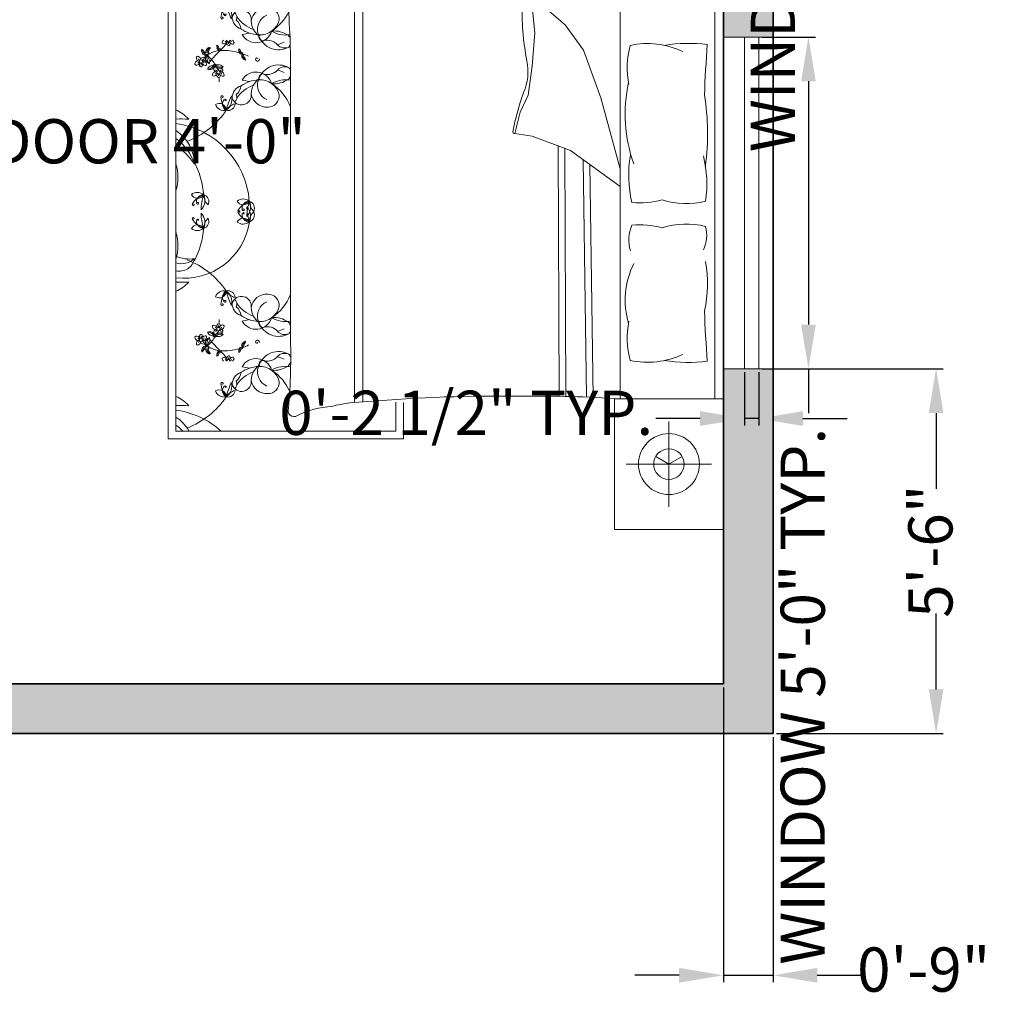
# Model space of a CAD drawing. Units: inches. Extents: x 2073 to 2646, y 2372 to 3017.
# Tile 2 of 8: x 2396 to 2572, y 2372 to 2550. Entities that reach past the tile are written whole.
import ezdxf

# ---------------------------------------------------------------- set-up
doc = ezdxf.new("R2010")
doc.units = ezdxf.units.IN
for name, color, linetype, lineweight in [('A-ANNO-DIMS', 2, 'Continuous', 18), ('A-FURN', 8, 'Continuous', 18), ('A-GLAZ', 4, 'Continuous', 18), ('A-WALL', 7, 'Continuous', 35), ('A-WALL-PATT', 30, 'Continuous', 13)]:
    doc.layers.add(name, color=color, linetype=linetype, lineweight=lineweight)
doc.styles.get("Standard").update_dxf_attribs({"font": 'arial.ttf'})
doc.dimstyles.new('ISO-25', dxfattribs={"dimtxt": 8, "dimasz": 8, "dimexe": 1.25, "dimexo": 0.625, "dimtad": 0, "dimdec": 1, "dimlunit": 4, "dimtxsty": 'Standard', "dimcen": 2.5, "dimadec": 0, "dimazin": 0, "dimtfac": 1, "dimtdec": 1, "dimtmove": 0, "dimatfit": 3, "dimfxl": 1, "dimarcsym": 0})

# ---------------------------------------------------------------- blocks, each defined once
blk = doc.blocks.new('bed')
at = {"color": 0}
for p, q in [((2249.53, 3172.75), (2367.64, 3172.75)), ((2273.15, 3172.75), (2273.15, 3140.33)), ((2261.34, 3155.19), (2261.34, 3170.62)), ((2344.02, 3171.23), (2273.15, 3171.23)), ((2355.83, 3155.19), (2355.83, 3170.62)), ((2269.06, 3162.9), (2253.62, 3162.9)), ((2348.11, 3162.9), (2363.55, 3162.9)), ((2273.15, 3154.08), (2344.02, 3154.08)), ((2289.56, 3150.57), (2302.44, 3154.08)), ((2305.6, 3154.08), (2299.13, 3145.07)), ((2280.95, 3147.46), (2289.56, 3150.57)), ((2343.7, 3149.18), (2301.65, 3148.59)), ((2276.4, 3144.12), (2280.95, 3147.46)), ((2343.66, 3147.96), (2300.77, 3147.36)), ((2272.09, 3139.1), (2276.4, 3144.12)), ((2299.13, 3145.07), (2296.5, 3138.14)), ((2343.59, 3144.24), (2298.75, 3144.07)), ((2343.6, 3143.03), (2298.28, 3142.85)), ((2273.05, 3138.14), (2272.09, 3139.1)), ((2277.84, 3138.62), (2273.05, 3138.14)), ((2283.82, 3138.14), (2277.84, 3138.62)), ((2289.08, 3137.42), (2283.82, 3138.14)), ((2292.19, 3135.99), (2289.08, 3137.42)), ((2296.5, 3138.14), (2296.02, 3135.03)), ((2296.02, 3135.03), (2292.19, 3135.99)), ((2265.12, 3114.85), (2271.8, 3114.85)), ((2265.12, 3072.3), (2265.12, 3114.85)), ((2271.8, 3113.48), (2266.49, 3113.48)), ((2266.49, 3113.48), (2266.49, 3073.67)), ((2349.86, 3113.48), (2344.65, 3113.48)), ((2344.68, 3114.85), (2351.23, 3114.85)), ((2349.86, 3073.67), (2349.86, 3113.48)), ((2351.23, 3114.85), (2351.23, 3072.3)), ((2344.56, 3107.48), (2271.79, 3107.48)), ((2344.67, 3106.01), (2271.79, 3106.01)), ((2332.56, 3094.41), (2284.61, 3094.41)), ((2278.13, 3085.65), (2277.87, 3086.98)), ((2286.38, 3085.65), (2286.64, 3086.98)), ((2329.96, 3085.65), (2329.7, 3086.98)), ((2338.22, 3085.65), (2338.48, 3086.98)), ((2266.49, 3073.67), (2349.86, 3073.67)), ((2351.23, 3072.3), (2265.12, 3072.3))]:
    blk.add_line(p, q, dxfattribs=at)
for points in [[(2273.15, 3153.06), (2249.53, 3153.06), (2249.53, 3172.75)], [(2344.02, 3172.75), (2344.02, 3153.06), (2367.64, 3153.06), (2367.64, 3172.75)], [(2261.34, 3162.9), (2262.72, 3165.29)], [(2355.83, 3162.9), (2354.45, 3165.29)], [(2261.34, 3162.9), (2262.72, 3160.52)], [(2355.83, 3162.9), (2354.45, 3160.52)]]:
    blk.add_lwpolyline(points, dxfattribs=at)
for points in [[(2279.94, 3169.8, 0.074897), (2280.08, 3162.09, -0.472817)], [(2308.03, 3161.66, 0.14099), (2308.27, 3169.53, 0.235245)], [(2313.08, 3161.66, -0.14099), (2312.84, 3169.53, -0.235245)], [(2337.23, 3169.8, -0.074897), (2337.09, 3162.09, 0.472817)], [(2271.85, 3128.28, 0.001242), (2271.79, 3105.87, -0.127202), (2269.42, 3094.7)], [(2344.52, 3108.41, 0.056112), (2345.38, 3101.91, 0.095341), (2347.04, 3095.66)]]:
    blk.add_lwpolyline(points, format="xyb", dxfattribs=at)
for centre, radius in [((2261.34, 3162.9), 5.51), ((2355.83, 3162.9), 5.51), ((2261.34, 3162.9), 2.76), ((2355.83, 3162.9), 2.76), ((2284.95, 3081.37), 0.301), ((2331.4, 3081.37), 0.301), ((2282.98, 3078.2), 0.301), ((2333.36, 3078.2), 0.301)]:
    blk.add_circle(centre, radius, dxfattribs=at)
for centre, radius, start, end in [((2345.04, 4293.82), 1125.9, 266.68521, 267.14978), ((2296.12, 3127.06), 42.84, 82.2196, 99.497), ((2305.17, 3148.71), 21.05, 81.5249, 103.96), ((2314.46, 3163.91), 5.84, 63.3437, 106.1026), ((2323.22, 3149.14), 20.76, 76.3427, 101.1841), ((2272.13, 4293.82), 1125.9, 272.85022, 273.31479), ((2294.98, 3158.99), 15.22, 155.1316, 191.7583), ((2322.19, 3158.99), 15.22, 348.2417, 24.8684), ((2294.11, 3157.71), 14.47, 354.0129, 15.8293), ((2327, 3157.71), 14.47, 164.1707, 185.9871), ((2292.48, 3182.44), 27.45, 258.0397, 289.2615), ((2303.6, 3176.44), 20.83, 259.8617, 283.6238), ((2315.25, 3161.88), 6.26, 245.0183, 288.5407), ((2326.19, 3170.02), 15.03, 243.8761, 286.1746), ((2284.15, 3171.19), 15.83, 255.1039, 281.0369), ((2333.02, 3171.19), 15.83, 258.9631, 284.8961), ((2555.75, 3139.65), 212.22, 176.1, 180.9282), ((2163.8, 3136.16), 108.33, 355.8294, 1.553), ((2274.12, 3180.92), 44.58, 267.4519, 281.3392), ((2284.77, 3127.79), 9.61, 66.2616, 101.3392), ((2304.22, 3179.66), 45.8, 250.1194, 259.3383), ((2295.75, 3134.94), 0.285, 268.8623, 19.7536), ((2620.36, 3131.93), 276.84, 179.1145, 184.8735), ((2346.15, 3095.06), 1.08, 246.5219, 33.8264), ((2270.51, 3094.78), 1.09, 183.98, 297.3412), ((2283.2, 2971.46), 122.95, 89.3433, 95.6887), ((2270.05, 3086.09), 8.94, 33.6671, 63.2997), ((2282.03, 3091.41), 4.56, 145.785, 184.7304), ((2273.33, 3093.53), 4.89, 328.8218, 9.1554), ((2279.39, 3093.1), 1.42, 120.0293, 142.325), ((2277.12, 3092.26), 3.76, 289.2822, 29.1751), ((2278.79, 3093.38), 1.77, 311.5653, 23.8354), ((2279.39, 3093.1), 1.42, 44.4517, 63.558), ((2287.39, 3092.26), 3.76, 150.8249, 250.7178), ((2285.72, 3093.38), 1.77, 156.1646, 228.4347), ((2285.12, 3093.1), 1.42, 113.229, 135.5483), ((2285.12, 3093.1), 1.42, 37.675, 66.7144), ((2282.48, 3091.41), 4.56, 355.2696, 34.215), ((2291.18, 3093.53), 4.89, 169.7133, 211.1782), ((2294.46, 3086.09), 8.94, 111.4941, 146.3329), ((2321.89, 3086.09), 8.94, 33.6671, 68.5059), ((2333.87, 3091.41), 4.56, 145.785, 184.7304), ((2325.17, 3093.53), 4.89, 328.8218, 10.2867), ((2331.23, 3093.1), 1.42, 113.2856, 142.325), ((2328.96, 3092.26), 3.76, 289.2822, 29.1751), ((2331.23, 3093.1), 1.42, 44.4517, 66.7144), ((2330.63, 3093.38), 1.77, 311.5653, 23.8354), ((2336.18, 2979.53), 114.93, 85.2402, 91.8035), ((2339.23, 3092.26), 3.76, 150.8249, 250.7178), ((2337.56, 3093.38), 1.77, 156.1646, 228.4347), ((2336.96, 3093.1), 1.42, 106.6343, 135.5483), ((2336.96, 3093.1), 1.42, 37.675, 72.5814), ((2334.32, 3091.41), 4.56, 355.2696, 34.215), ((2343.02, 3093.53), 4.89, 169.249, 211.1782), ((2346.3, 3086.09), 8.94, 113.6453, 146.3329), ((2275.26, 3090.38), 1.99, 84.4856, 181.0538), ((2274.65, 3088.91), 3.55, 355.2933, 76.921), ((2281.57, 3090.25), 2.42, 131.5653, 195.1471), ((2276.55, 3091.58), 3.4, 7.436, 29.9149), ((2282.94, 3090.25), 2.42, 344.8529, 48.4347), ((2287.96, 3091.58), 3.4, 150.0851, 172.564), ((2289.86, 3088.91), 3.55, 103.079, 184.7067), ((2289.25, 3090.38), 1.99, 358.9462, 95.5144), ((2327.09, 3090.38), 1.99, 84.4856, 181.0538), ((2326.48, 3088.91), 3.55, 355.2933, 76.921), ((2333.4, 3090.25), 2.42, 131.5653, 195.1471), ((2328.39, 3091.58), 3.4, 7.436, 29.9149), ((2334.78, 3090.25), 2.42, 344.8529, 48.4347), ((2339.8, 3091.58), 3.4, 150.0851, 172.564), ((2341.7, 3088.91), 3.55, 103.079, 184.7067), ((2341.09, 3090.38), 1.99, 358.9462, 95.5144), ((2276.08, 3090.1), 2.82, 174.9449, 262.8857), ((2277.18, 3091.17), 2.74, 201.5819, 291.4221), ((2276.66, 3088.19), 2.94, 299.9085, 73.1337), ((2287.85, 3088.19), 2.94, 106.8663, 240.0915), ((2287.32, 3091.17), 2.74, 248.5779, 338.4181), ((2288.43, 3090.1), 2.82, 277.1143, 5.0551), ((2327.91, 3090.1), 2.82, 174.9449, 262.8857), ((2329.02, 3091.17), 2.74, 201.5819, 291.4221), ((2328.5, 3088.19), 2.94, 299.9085, 73.1337), ((2339.68, 3088.19), 2.94, 106.8663, 240.0915), ((2339.16, 3091.17), 2.74, 248.5779, 338.4181), ((2340.27, 3090.1), 2.82, 277.1143, 5.0551), ((2275.58, 3090.72), 3.43, 272.3591, 324.0401), ((2271.86, 3089), 6.34, 326.2883, 356.5076), ((2282.03, 3091.41), 4.56, 212.7011, 216.3445), ((2278.52, 3089.43), 0.733, 257.3041, 15.1471), ((2282.59, 3088.31), 0.228, 102.7051, 280.4384), ((2282.57, 3088.45), 0.37, 280.4384, 100.4136), ((2285.99, 3089.43), 0.733, 164.8529, 282.6959), ((2282.48, 3091.41), 4.56, 323.6555, 327.2989), ((2288.92, 3090.72), 3.43, 215.9599, 267.6409), ((2292.65, 3089), 6.34, 183.4924, 213.7117), ((2327.42, 3090.72), 3.43, 272.3591, 324.0401), ((2323.7, 3089), 6.34, 326.2883, 356.5076), ((2333.87, 3091.41), 4.56, 212.7011, 216.3445), ((2330.36, 3089.43), 0.733, 257.3041, 15.1471), ((2333.78, 3088.45), 0.37, 79.5864, 259.5616), ((2333.75, 3088.31), 0.228, 259.5616, 77.2949), ((2337.82, 3089.43), 0.733, 164.8529, 282.6959), ((2334.32, 3091.41), 4.56, 323.6555, 327.2989), ((2340.76, 3090.72), 3.43, 215.9599, 267.6409), ((2344.49, 3089), 6.34, 183.4924, 213.7117), ((2275.43, 3085.55), 1.77, 80.264, 250.8688), ((2271.91, 3089.45), 5.58, 301.2614, 341.7045), ((2290.78, 3082.37), 9.78, 153.0032, 159.8941), ((2292.6, 3089.45), 5.58, 198.2955, 238.7386), ((2289.08, 3085.55), 1.77, 289.1312, 99.736), ((2309.5, 3071.59), 15.42, 94.4623, 172.255), ((2309.57, 3085.82), 1.71, 137.7873, 219.1145), ((2307.63, 3085.87), 1.29, 298.5391, 58.3627), ((2309.53, 3086.61), 1.28, 63.0274, 163.8037), ((2308.24, 3089.6), 2.63, 271.4585, 315.3727), ((2309.31, 3084.75), 2.44, 45.5411, 114.3101), ((2311.53, 3097.27), 10.79, 252.593, 267.2582), ((2309.56, 3086.92), 1.26, 177.7585, 283.852), ((2311.99, 3088.23), 3.9, 198.9159, 238.011), ((2310.98, 3084.75), 2.44, 65.6899, 134.4589), ((2308.75, 3097.27), 10.79, 272.7418, 287.407), ((2310.75, 3086.61), 1.28, 16.1963, 116.9726), ((2312.05, 3089.6), 2.63, 224.6273, 268.5415), ((2308.29, 3088.23), 3.9, 301.989, 341.0841), ((2310.72, 3086.92), 1.26, 256.148, 2.2415), ((2312.66, 3085.87), 1.29, 121.6373, 241.4609), ((2310.71, 3085.82), 1.71, 320.8855, 42.2127), ((2310.28, 3075.15), 11.94, 352.8636, 81.8197), ((2327.26, 3085.55), 1.77, 80.264, 250.8688), ((2323.75, 3089.45), 5.58, 301.2614, 341.7045), ((2325.57, 3082.37), 9.78, 20.1059, 26.9968), ((2344.44, 3089.45), 5.58, 198.2955, 238.7386), ((2340.92, 3085.55), 1.77, 289.1312, 99.736), ((2275, 3086.08), 2.21, 265.969, 344.3045), ((2277.38, 3083.14), 2.36, 96.1662, 141.5825), ((2281.29, 3084.79), 0.62, 101.3256, 154.4621), ((2280.4, 3086.9), 1.87, 280.2588, 300.656), ((2280.83, 3088.39), 3.33, 268.3264, 277.1302), ((2290.78, 3082.37), 9.78, 163.5842, 183.8277), ((2279.99, 3086.89), 1.9, 308.2101, 316.3071), ((2281.16, 3085.65), 0.567, 278.3432, 4.2869), ((2280.84, 3086.14), 0.99, 300.656, 332.6341), ((2281.59, 3085.49), 0.241, 55.7657, 157.4417), ((2281.96, 3085.71), 0.241, 84.3784, 186.0543), ((2281.74, 3086.68), 0.99, 269.1859, 301.164), ((2282.03, 3086.17), 0.567, 237.5332, 323.4768), ((2281.48, 3087.78), 1.9, 285.5129, 293.6099), ((2282.72, 3085.65), 0.62, 87.3579, 140.4944), ((2281.28, 3087.43), 1.87, 301.164, 321.5612), ((2279.77, 3087.76), 3.33, 324.6898, 333.4936), ((2287.12, 3083.14), 2.36, 38.4175, 83.8338), ((2289.51, 3086.08), 2.21, 195.6955, 274.031), ((2309.83, 3085.86), 0.167, 283.852, 219.9245), ((2310.03, 3085.09), 0.192, 238.011, 71.5592), ((2310.06, 3085.18), 0.093, 71.5592, 188.0167), ((2310.25, 3085.09), 0.192, 108.4408, 301.989), ((2310.22, 3085.18), 0.093, 351.9833, 108.4408), ((2310.44, 3085.92), 0.101, 320.1909, 256.0209), ((2326.84, 3086.08), 2.21, 265.969, 344.3045), ((2329.22, 3083.14), 2.36, 96.1662, 141.5825), ((2335.06, 3087.43), 1.87, 218.4388, 238.836), ((2333.63, 3085.65), 0.62, 39.5056, 92.6421), ((2336.58, 3087.76), 3.33, 206.5064, 215.3102), ((2334.32, 3086.17), 0.567, 216.5232, 302.4668), ((2334.61, 3086.68), 0.99, 238.836, 270.8141), ((2334.87, 3087.78), 1.9, 246.3901, 254.4871), ((2334.38, 3085.71), 0.241, 353.9457, 95.6216), ((2334.76, 3085.49), 0.241, 22.5583, 124.2343), ((2335.19, 3085.65), 0.567, 175.7131, 261.6568), ((2335.5, 3086.14), 0.99, 207.3659, 239.344), ((2325.57, 3082.37), 9.78, 356.1723, 16.4158), ((2336.35, 3086.89), 1.9, 223.6929, 231.7899), ((2335.95, 3086.9), 1.87, 239.344, 259.7412), ((2335.52, 3088.39), 3.33, 262.8698, 271.6736), ((2335.06, 3084.79), 0.62, 25.5379, 78.6744), ((2341.35, 3086.08), 2.21, 195.6955, 274.031), ((2338.96, 3083.14), 2.36, 38.4175, 83.8338), ((2273.92, 3083.1), 1.28, 92.9516, 193.728), ((2271.31, 3085.04), 2.63, 301.3827, 345.2969), ((2274.66, 3081.37), 2.44, 75.4653, 144.2343), ((2270.34, 3093.33), 10.79, 282.5173, 297.1824), ((2275.06, 3083.63), 1.09, 63.9755, 143.2681), ((2279.54, 3083.62), 0.502, 101.5637, 142.6358), ((2279.12, 3083.15), 0.301, 273.2768, 86.7232), ((2279.47, 3083.44), 0.287, 91.1081, 181.8675), ((2279.78, 3082.86), 0.622, 80.3487, 133.6538), ((2279.66, 3083.37), 0.492, 229.7889, 317.6792), ((2279.13, 3084.01), 0.723, 288.7263, 352.5032), ((2279.66, 3082.21), 0.985, 83.0852, 105.7171), ((2279.63, 3083.98), 0.232, 345.2356, 144.9248), ((2279.84, 3083.22), 0.259, 317.6792, 80.3487), ((2289.45, 3083.63), 1.09, 36.7319, 116.0245), ((2289.85, 3081.37), 2.44, 35.7657, 104.5347), ((2294.17, 3093.33), 10.79, 242.8176, 257.4827), ((2290.59, 3083.1), 1.28, 346.272, 87.0484), ((2293.2, 3085.04), 2.63, 194.7031, 238.6173), ((2325.76, 3083.1), 1.28, 92.9516, 193.728), ((2323.15, 3085.04), 2.63, 301.3827, 345.2969), ((2326.5, 3081.37), 2.44, 75.4653, 144.2343), ((2322.18, 3093.33), 10.79, 282.5173, 297.1824), ((2326.9, 3083.63), 1.09, 63.9755, 143.2681), ((2336.51, 3083.22), 0.259, 99.6513, 222.3208), ((2336.68, 3083.37), 0.492, 222.3208, 310.2111), ((2336.57, 3082.86), 0.622, 46.3462, 99.6513), ((2336.72, 3083.98), 0.232, 35.0752, 194.7644), ((2337.21, 3084.01), 0.723, 187.4968, 251.2737), ((2336.69, 3082.21), 0.985, 74.2829, 96.9148), ((2336.88, 3083.44), 0.287, 358.1325, 88.8919), ((2336.81, 3083.62), 0.502, 37.3642, 78.4363), ((2337.23, 3083.15), 0.301, 93.2768, 266.7232), ((2341.29, 3083.63), 1.09, 36.7319, 116.0245), ((2341.69, 3081.37), 2.44, 35.7657, 104.5347), ((2346, 3093.33), 10.79, 242.8176, 257.4827), ((2345.04, 3085.04), 2.63, 194.7031, 238.6173), ((2342.42, 3083.1), 1.28, 346.272, 87.0484), ((2255.01, 3071.59), 15.42, 7.745, 41.8856), ((2281.39, 3070.07), 15.42, 124.3865, 158.5908), ((2274.35, 3082.43), 1.71, 167.7115, 249.0387), ((2272.64, 3081.51), 1.29, 328.4633, 88.2869), ((2275.25, 3085.73), 3.9, 228.8402, 267.9352), ((2273.8, 3083.38), 1.26, 207.6827, 313.7762), ((2274.56, 3082.59), 0.167, 313.7762, 249.7183), ((2275.1, 3082.12), 0.093, 101.4834, 217.9409), ((2275.12, 3082.03), 0.192, 267.9352, 101.4834), ((2279.53, 3082.6), 0.497, 217.7621, 259.0403), ((2280.07, 3083.26), 0.913, 203.4276, 227.6104), ((2279.11, 3082.33), 0.699, 355.053, 68.3618), ((2279.58, 3082.29), 0.231, 232.4737, 355.053), ((2272.84, 3074.04), 11.21, 43.1541, 52.0459), ((2280.59, 3080.82), 0.62, 101.3256, 154.4621), ((2279.69, 3082.92), 1.87, 280.2588, 300.656), ((2279.29, 3082.92), 1.9, 308.2101, 316.3071), ((2280.45, 3081.67), 0.567, 278.3432, 4.2869), ((2280.14, 3082.17), 0.99, 300.656, 332.6341), ((2280.88, 3081.52), 0.241, 55.7657, 157.4417), ((2285.91, 3082.12), 4.9, 184.756, 209.2041), ((2292.97, 3092.56), 16.14, 222.2412, 232.1744), ((2283.38, 3081.51), 0.833, 272.8499, 356.1226), ((2282.65, 3081.81), 1.37, 304.5369, 16.3699), ((2282.79, 3081.18), 0.807, 321.7607, 7.9252), ((2284.55, 3081.43), 0.97, 127.3105, 187.9252), ((2283.22, 3081.54), 0.996, 355.0106, 41.658), ((2284.87, 3080.46), 0.948, 104.7558, 148.0499), ((2284.62, 3081.78), 0.41, 126.1046, 271.4281), ((2284.57, 3081.9), 0.295, 353.7526, 131.7054), ((2284.3, 3081.55), 0.414, 0.0645, 61.1507), ((2284.39, 3081.9), 0.473, 311.8413, 355.7877), ((2285.37, 3081.83), 0.502, 101.5637, 176.365), ((2285.3, 3081.65), 0.287, 91.1081, 181.8675), ((2285.61, 3081.07), 0.622, 80.3487, 133.6538), ((2285.5, 3081.59), 0.492, 229.7889, 317.6792), ((2284.96, 3082.22), 0.723, 288.7263, 352.5032), ((2285.49, 3080.43), 0.985, 83.0852, 105.7171), ((2285.46, 3082.19), 0.232, 345.2356, 144.9248), ((2285.67, 3081.43), 0.259, 317.6792, 80.3487), ((2286.41, 3075.61), 5.88, 87.1071, 94.7585), ((2289.39, 3082.03), 0.192, 78.5166, 272.0648), ((2289.26, 3085.73), 3.9, 272.0648, 311.1598), ((2289.41, 3082.12), 0.093, 322.0591, 78.5166), ((2290.71, 3083.38), 1.26, 226.2238, 332.3173), ((2289.97, 3082.66), 0.101, 290.2667, 226.2271), ((2291.87, 3081.51), 1.29, 91.7131, 211.5367), ((2290.16, 3082.43), 1.71, 290.9613, 12.2885), ((2283.12, 3070.07), 15.42, 21.4092, 55.6135), ((2333.23, 3070.07), 15.42, 124.3865, 158.5908), ((2326.19, 3082.43), 1.71, 167.7115, 249.0387), ((2325.64, 3083.38), 1.26, 207.6827, 313.7762), ((2327.09, 3085.73), 3.9, 228.8402, 267.9352), ((2324.48, 3081.51), 1.29, 328.4633, 88.2869), ((2326.39, 3082.59), 0.167, 313.7762, 249.7183), ((2326.93, 3082.12), 0.093, 101.4834, 217.9409), ((2326.95, 3082.03), 0.192, 267.9352, 101.4834), ((2329.94, 3075.61), 5.88, 85.2415, 92.8929), ((2330.68, 3081.43), 0.259, 99.6513, 222.3208), ((2330.85, 3081.59), 0.492, 222.3208, 310.2111), ((2330.74, 3081.07), 0.622, 46.3462, 99.6513), ((2330.89, 3082.19), 0.232, 35.0752, 194.7644), ((2331.38, 3082.22), 0.723, 187.4968, 251.2737), ((2330.86, 3080.43), 0.985, 74.2829, 96.9148), ((2331.05, 3081.65), 0.287, 358.1325, 88.8919), ((2330.98, 3081.83), 0.502, 3.635, 78.4363), ((2331.77, 3081.9), 0.295, 48.2946, 186.2474), ((2331.95, 3081.9), 0.473, 184.2123, 228.1587), ((2332.05, 3081.55), 0.414, 118.8493, 179.9355), ((2331.73, 3081.78), 0.41, 268.5719, 53.8954), ((2331.48, 3080.46), 0.948, 31.9501, 75.2442), ((2333.13, 3081.54), 0.996, 138.342, 184.9894), ((2332.97, 3081.51), 0.833, 183.8774, 267.1501), ((2333.7, 3081.81), 1.37, 163.6301, 235.4631), ((2331.79, 3081.43), 0.97, 352.0748, 52.6895), ((2333.55, 3081.18), 0.807, 172.0748, 218.2393), ((2323.38, 3092.56), 16.14, 307.8256, 317.7588), ((2330.44, 3082.12), 4.9, 330.7959, 355.244), ((2343.51, 3074.04), 11.21, 127.9541, 136.8459), ((2335.46, 3081.52), 0.241, 22.5583, 124.2343), ((2335.89, 3081.67), 0.567, 175.7131, 261.6568), ((2336.21, 3082.17), 0.99, 207.3659, 239.344), ((2337.06, 3082.92), 1.9, 223.6929, 231.7899), ((2336.65, 3082.92), 1.87, 239.344, 259.7412), ((2335.76, 3080.82), 0.62, 25.5379, 78.6744), ((2337.24, 3082.33), 0.699, 111.6382, 184.947), ((2336.77, 3082.29), 0.231, 184.947, 307.5263), ((2336.28, 3083.26), 0.913, 312.3896, 336.5724), ((2336.82, 3082.6), 0.497, 280.9597, 322.2379), ((2341.23, 3082.03), 0.192, 78.5166, 272.0648), ((2341.1, 3085.73), 3.9, 272.0648, 311.1598), ((2341.25, 3082.12), 0.093, 322.0591, 78.5166), ((2342.55, 3083.38), 1.26, 226.2238, 332.3173), ((2341.81, 3082.66), 0.101, 290.2667, 226.2271), ((2343.7, 3081.51), 1.29, 91.7131, 211.5367), ((2341.99, 3082.43), 1.71, 290.9613, 12.2885), ((2334.95, 3070.07), 15.42, 21.4092, 55.6135), ((2361.34, 3071.59), 15.42, 138.1144, 172.255), ((2280.12, 3084.42), 3.33, 268.3264, 277.1302), ((2280.79, 3079.73), 0.336, 146.8636, 236.9021), ((2285.53, 3087.13), 8.79, 235.1882, 238.8844), ((2281.37, 3080.22), 0.909, 199.4799, 267.6828), ((2281.17, 3079.91), 0.348, 238.8844, 314.2646), ((2281.59, 3079.27), 0.262, 19.3605, 201.7548), ((2281.59, 3079.47), 0.262, 311.8703, 134.2646), ((2282.36, 3080.66), 1.37, 247.2305, 319.0635), ((2281.9, 3080.2), 0.807, 264.4544, 310.6188), ((2286.41, 3075.61), 5.88, 120.544, 139.818), ((2283.06, 3078.85), 0.97, 70.0041, 130.6188), ((2282.43, 3080.03), 0.996, 297.7043, 344.3516), ((2282.96, 3080.02), 0.807, 8.7227, 54.8872), ((2283, 3079.38), 1.37, 0.278, 72.111), ((2283.62, 3079.88), 0.833, 20.5253, 88.5375), ((2284.72, 3080.29), 0.97, 188.7227, 249.3375), ((2284.32, 3080.8), 0.298, 148.0499, 225.6268), ((2286.41, 3075.61), 5.88, 113.0501, 113.8477), ((2284.34, 3081.14), 0.594, 247.4086, 351.4386), ((2283.47, 3079.81), 0.996, 334.9899, 21.6373), ((2284.51, 3081.11), 0.199, 262.906, 7.132), ((2285.36, 3080.81), 0.497, 151.2196, 259.0403), ((2285.9, 3081.47), 0.913, 203.4276, 227.6104), ((2284.94, 3080.54), 0.699, 355.053, 68.3618), ((2285.41, 3080.5), 0.231, 232.4737, 355.053), ((2308.35, 3078.35), 1.28, 63.0274, 163.8037), ((2307.06, 3081.34), 2.63, 271.4585, 315.3727), ((2311.93, 3078.35), 1.28, 16.1963, 116.9726), ((2313.23, 3081.34), 2.63, 224.6273, 268.5415), ((2331.41, 3080.54), 0.699, 111.6382, 184.947), ((2330.94, 3080.5), 0.231, 184.947, 307.5263), ((2330.45, 3081.47), 0.913, 312.3896, 336.5724), ((2330.99, 3080.81), 0.497, 280.9597, 28.7804), ((2332.01, 3081.14), 0.594, 188.5614, 292.5914), ((2331.84, 3081.11), 0.199, 172.868, 277.094), ((2332.87, 3079.81), 0.996, 158.3627, 205.0101), ((2332.73, 3079.88), 0.833, 91.4625, 159.4747), ((2333.34, 3079.38), 1.37, 107.889, 179.722), ((2331.63, 3080.29), 0.97, 290.6625, 351.2773), ((2329.94, 3075.61), 5.88, 66.1523, 66.9499), ((2332.03, 3080.8), 0.298, 314.3732, 31.9501), ((2333.39, 3080.02), 0.807, 125.1128, 171.2773), ((2329.94, 3075.61), 5.88, 40.182, 59.456), ((2333.29, 3078.85), 0.97, 49.3812, 109.9959), ((2333.99, 3080.66), 1.37, 220.9365, 292.7695), ((2333.91, 3080.03), 0.996, 195.6484, 242.2957), ((2334.44, 3080.2), 0.807, 229.3812, 275.5456), ((2334.75, 3079.47), 0.262, 45.7354, 228.1297), ((2334.75, 3079.27), 0.262, 338.2452, 160.6395), ((2335.18, 3079.91), 0.348, 225.7354, 301.1156), ((2334.98, 3080.22), 0.909, 272.3172, 340.5201), ((2330.82, 3087.13), 8.79, 301.1156, 304.8118), ((2335.55, 3079.73), 0.336, 303.0979, 33.1364), ((2336.22, 3084.42), 3.33, 262.8698, 271.6736), ((2281.27, 3079.88), 0.783, 212.8155, 277.3992), ((2280.81, 3079.35), 0.909, 266.9701, 338.2913), ((2276.02, 3085.84), 8.79, 302.6784, 306.3746), ((2281.04, 3078.63), 0.336, 214.3538, 304.3923), ((2281.09, 3079.13), 0.783, 280.3057, 17.1958), ((2281.03, 3079.05), 0.348, 306.3746, 21.7548), ((2286.53, 3077.08), 5.24, 153.7819, 158.2913), ((2285.91, 3082.12), 4.9, 214.0033, 222.4917), ((2282.49, 3079.88), 0.833, 218.3208, 298.8162), ((2282.35, 3077.63), 0.298, 148.0499, 225.6268), ((2282.9, 3077.29), 0.948, 104.7558, 148.0499), ((2282.37, 3077.97), 0.594, 247.4086, 351.4386), ((2282.65, 3078.61), 0.41, 126.1046, 271.4281), ((2282.61, 3078.72), 0.295, 353.7526, 131.7054), ((2282.54, 3077.94), 0.199, 262.906, 7.132), ((2282.33, 3078.37), 0.414, 0.0645, 61.1507), ((2282.43, 3078.73), 0.473, 311.8413, 355.7877), ((2283.4, 3078.66), 0.502, 101.5637, 176.365), ((2283.39, 3077.64), 0.497, 151.2196, 259.0403), ((2283.33, 3078.48), 0.287, 91.1081, 181.8675), ((2283.93, 3078.3), 0.913, 203.4276, 227.6104), ((2283.64, 3077.9), 0.622, 80.3487, 133.6538), ((2283.53, 3078.42), 0.492, 229.7889, 317.6792), ((2283, 3079.05), 0.723, 288.7263, 352.5032), ((2282.97, 3077.37), 0.699, 355.053, 68.3618), ((2283.52, 3077.26), 0.985, 83.0852, 105.7171), ((2283.49, 3079.02), 0.232, 345.2356, 144.9248), ((2283.7, 3078.26), 0.259, 317.6792, 80.3487), ((2308.32, 3063.33), 15.42, 94.4623, 117.4146), ((2308.39, 3077.56), 1.71, 137.7873, 219.1145), ((2306.45, 3077.61), 1.29, 298.5391, 58.3627), ((2308.13, 3076.49), 2.44, 45.5411, 114.3101), ((2310.81, 3079.97), 3.9, 198.9159, 238.011), ((2310.35, 3089), 10.79, 252.593, 267.2582), ((2308.38, 3078.66), 1.26, 177.7585, 283.852), ((2308.65, 3077.6), 0.167, 283.852, 219.9245), ((2312.16, 3076.49), 2.44, 65.6899, 134.4589), ((2309.93, 3089), 10.79, 272.7418, 287.407), ((2311.62, 3077.66), 0.101, 320.1909, 256.0209), ((2309.47, 3079.97), 3.9, 301.989, 341.0841), ((2311.9, 3078.66), 1.26, 256.148, 2.2415), ((2313.84, 3077.61), 1.29, 121.6373, 241.4609), ((2311.89, 3077.56), 1.71, 320.8855, 42.2127), ((2311.96, 3063.33), 15.42, 62.5854, 85.5377), ((2332.65, 3078.26), 0.259, 99.6513, 222.3208), ((2332.82, 3078.42), 0.492, 222.3208, 310.2111), ((2332.71, 3077.9), 0.622, 46.3462, 99.6513), ((2332.86, 3079.02), 0.232, 35.0752, 194.7644), ((2333.35, 3079.05), 0.723, 187.4968, 251.2737), ((2333.37, 3077.37), 0.699, 111.6382, 184.947), ((2332.83, 3077.26), 0.985, 74.2829, 96.9148), ((2333.01, 3078.48), 0.287, 358.1325, 88.8919), ((2332.42, 3078.3), 0.913, 312.3896, 336.5724), ((2332.95, 3078.66), 0.502, 3.635, 78.4363), ((2332.95, 3077.64), 0.497, 280.9597, 28.7804), ((2333.98, 3077.97), 0.594, 188.5614, 292.5914), ((2333.85, 3079.88), 0.833, 241.1838, 321.6792), ((2333.74, 3078.72), 0.295, 48.2946, 186.2474), ((2333.92, 3078.73), 0.473, 184.2123, 228.1587), ((2334.02, 3078.37), 0.414, 118.8493, 179.9355), ((2333.81, 3077.94), 0.199, 172.868, 277.094), ((2333.7, 3078.61), 0.41, 268.5719, 53.8954), ((2333.44, 3077.29), 0.948, 31.9501, 75.2442), ((2330.44, 3082.12), 4.9, 317.5083, 325.9967), ((2334, 3077.63), 0.298, 314.3732, 31.9501), ((2335.25, 3079.13), 0.783, 162.8042, 259.6943), ((2329.82, 3077.08), 5.24, 21.7087, 26.2181), ((2335.53, 3079.35), 0.909, 201.7087, 273.0299), ((2335.32, 3079.05), 0.348, 158.2452, 233.6254), ((2335.08, 3079.88), 0.783, 262.6008, 327.1845), ((2340.32, 3085.84), 8.79, 233.6254, 237.3216), ((2335.3, 3078.63), 0.336, 235.6077, 325.6462), ((2262.74, 3069.53), 7.52, 33.4617, 60.1116), ((2266.95, 3071.27), 6.27, 22.5547, 48.9546), ((2249.77, 3074.64), 21.34, 357.4081, 3.6519), ((2283.44, 3077.33), 0.231, 232.4737, 355.053), ((2297.56, 3071.27), 6.27, 131.0454, 157.4453), ((2314.73, 3074.64), 21.34, 176.3481, 182.5919), ((2301.77, 3069.53), 7.52, 91.272, 146.5383), ((2304.47, 3068.13), 9.37, 107.8504, 143.6964), ((2309.39, 3065.49), 13.93, 124.0123, 144.053), ((2308.85, 3076.83), 0.192, 238.011, 71.5592), ((2308.88, 3076.92), 0.093, 71.5592, 188.0167), ((2311.44, 3076.83), 0.192, 108.4408, 301.989), ((2311.4, 3076.92), 0.093, 351.9833, 108.4408), ((2311.82, 3076.24), 6.91, 338.117, 6.6195), ((2318.16, 3074.32), 2.77, 346.3898, 79.0739), ((2316.08, 3074.7), 3.5, 342.8609, 41.9049), ((2301.61, 3074.64), 21.34, 357.4081, 3.6519), ((2318.79, 3071.27), 6.27, 22.5547, 48.9546), ((2332.91, 3077.33), 0.231, 184.947, 307.5263), ((2349.39, 3071.27), 6.27, 131.0454, 157.4453), ((2366.57, 3074.64), 21.34, 176.3481, 182.5919), ((2353.6, 3069.53), 7.52, 119.8884, 146.5383), ((2260.04, 3068.13), 9.37, 36.3036, 46.4814), ((2356.31, 3068.13), 9.37, 133.5186, 143.6964), ((2304.01, 3065.56), 8.48, 73.5431, 107.0202), ((2307.37, 3061.19), 12.54, 94.3787, 95.6357), ((2313.97, 3052.6), 22.41, 109.7217, 109.9028), ((2316.27, 3065.56), 8.48, 72.9798, 106.4569), ((2312.91, 3061.19), 12.54, 84.3643, 85.6213), ((2306.31, 3052.6), 22.41, 70.0972, 70.2783)]:
    blk.add_arc(centre, radius, start, end, dxfattribs=at)
blk = doc.blocks.new('GLAZ-60IN')
for p, q in [((0, 60), (0, 0)), ((2.6, 60), (2.6, 0))]:
    blk.add_line(p, q)
blk = doc.blocks.new('*D25')
at = {"layer": 'A-ANNO-DIMS', "color": 0, "lineweight": -2, "transparency": 16777216}
for p, q in [((2530.32, 2546.66), (2539.94, 2546.66)), ((2538.69, 2538.66), (2538.69, 2494.66)), ((2530.32, 2486.66), (2539.94, 2486.66)), ((2538.69, 2486.66), (2538.69, 2478.66))]:
    blk.add_line(p, q, dxfattribs=at)
at = {"layer": 'A-ANNO-DIMS', "color": 0, "transparency": 16777216}
for points in [[(2537.36, 2538.66), (2540.02, 2538.66), (2538.69, 2546.66)], [(2537.36, 2494.66), (2540.02, 2494.66), (2538.69, 2486.66)]]:
    blk.add_solid(points, dxfattribs=at)
at = {"layer": 'Defpoints', "color": 0, "transparency": 16777216}
for p in [(2529.69, 2546.66), (2529.69, 2486.66), (2538.69, 2486.66)]:
    blk.add_point(p, dxfattribs=at)
at = {"layer": 'A-ANNO-DIMS', "color": 0, "transparency": 16777216, "insert": (2538.69, 2427.42), "char_height": 8, "attachment_point": 5, "rotation": 90}
blk.add_mtext('WINDOW 5\'-0" TYP.', dxfattribs=at)
blk = doc.blocks.new('*D26')
at = {"layer": 'A-ANNO-DIMS', "color": 0, "lineweight": -2, "transparency": 16777216}
for p, q in [((2527.09, 2486.04), (2527.09, 2476.41)), ((2529.69, 2486.04), (2529.69, 2476.41)), ((2519.09, 2477.66), (2511.09, 2477.66)), ((2529.69, 2477.66), (2527.09, 2477.66)), ((2537.69, 2477.66), (2545.69, 2477.66))]:
    blk.add_line(p, q, dxfattribs=at)
at = {"layer": 'A-ANNO-DIMS', "color": 0, "transparency": 16777216}
for points in [[(2519.09, 2479), (2519.09, 2476.33), (2527.09, 2477.66)], [(2537.69, 2479), (2537.69, 2476.33), (2529.69, 2477.66)]]:
    blk.add_solid(points, dxfattribs=at)
at = {"layer": 'Defpoints', "color": 0, "transparency": 16777216}
for p in [(2527.09, 2486.66), (2529.69, 2486.66), (2527.09, 2477.66)]:
    blk.add_point(p, dxfattribs=at)
at = {"layer": 'A-ANNO-DIMS', "color": 0, "transparency": 16777216, "insert": (2476.76, 2477.66), "char_height": 8, "attachment_point": 5}
blk.add_mtext('0\'-2 1/2" TYP.', dxfattribs=at)
blk = doc.blocks.new('*D27')
at = {"layer": 'A-ANNO-DIMS', "color": 0, "lineweight": -2, "transparency": 16777216}
for p, q in [((2530.32, 2657.66), (2534.54, 2657.66)), ((2533.29, 2649.66), (2533.29, 2641.66)), ((2530.32, 2633.66), (2534.54, 2633.66)), ((2533.29, 2633.66), (2533.29, 2625.66))]:
    blk.add_line(p, q, dxfattribs=at)
at = {"layer": 'A-ANNO-DIMS', "color": 0, "transparency": 16777216}
for points in [[(2531.96, 2649.66), (2534.62, 2649.66), (2533.29, 2657.66)], [(2531.96, 2641.66), (2534.62, 2641.66), (2533.29, 2633.66)]]:
    blk.add_solid(points, dxfattribs=at)
at = {"layer": 'Defpoints', "color": 0, "transparency": 16777216}
for p in [(2529.69, 2657.66), (2529.69, 2633.66), (2533.29, 2633.66)]:
    blk.add_point(p, dxfattribs=at)
at = {"layer": 'A-ANNO-DIMS', "color": 0, "transparency": 16777216, "insert": (2533.29, 2574.42), "char_height": 8, "attachment_point": 5, "rotation": 90}
blk.add_mtext('WINDOW 2\'-0" TYP.', dxfattribs=at)
blk = doc.blocks.new('*D29')
at = {"layer": 'A-ANNO-DIMS', "color": 0, "lineweight": -2, "transparency": 16777216}
for p, q in [((2372.17, 2524.43), (2372.17, 2532.43)), ((2366.13, 2524.43), (2373.42, 2524.43)), ((2372.17, 2487.96), (2372.17, 2516.43)), ((2366.13, 2479.96), (2373.42, 2479.96))]:
    blk.add_line(p, q, dxfattribs=at)
at = {"layer": 'A-ANNO-DIMS', "color": 0, "transparency": 16777216}
for points in [[(2370.84, 2516.43), (2373.51, 2516.43), (2372.17, 2524.43)], [(2370.84, 2487.96), (2373.51, 2487.96), (2372.17, 2479.96)]]:
    blk.add_solid(points, dxfattribs=at)
at = {"layer": 'Defpoints', "color": 0, "transparency": 16777216}
for p in [(2365.5, 2524.43), (2372.17, 2524.43), (2365.5, 2479.96)]:
    blk.add_point(p, dxfattribs=at)
at = {"layer": 'A-ANNO-DIMS', "color": 0, "transparency": 16777216, "insert": (2372.17, 2595.59), "char_height": 8, "attachment_point": 5, "rotation": 90}
blk.add_mtext('CONSOLE 3\'-8 1/2" TYP.', dxfattribs=at)
blk = doc.blocks.new('*D41')
at = {"layer": 'A-ANNO-DIMS', "color": 0, "lineweight": -2, "transparency": 16777216}
for p, q in [((2295.23, 2520.2), (2295.23, 2528.03)), ((2343.29, 2520.2), (2343.29, 2528.03)), ((2303.23, 2526.78), (2335.29, 2526.78)), ((2343.29, 2526.78), (2351.29, 2526.78))]:
    blk.add_line(p, q, dxfattribs=at)
at = {"layer": 'A-ANNO-DIMS', "color": 0, "transparency": 16777216}
for points in [[(2303.23, 2528.12), (2303.23, 2525.45), (2295.23, 2526.78)], [(2335.29, 2528.12), (2335.29, 2525.45), (2343.29, 2526.78)]]:
    blk.add_solid(points, dxfattribs=at)
at = {"layer": 'Defpoints', "color": 0, "transparency": 16777216}
for p in [(2343.29, 2526.78), (2295.23, 2519.57), (2343.29, 2519.57)]:
    blk.add_point(p, dxfattribs=at)
at = {"layer": 'A-ANNO-DIMS', "color": 0, "transparency": 16777216, "insert": (2401.15, 2526.78), "char_height": 8, "attachment_point": 5}
blk.add_mtext('ENTRY DOOR 4\'-0"', dxfattribs=at)
blk = doc.blocks.new('*D46')
at = {"layer": 'A-ANNO-DIMS', "color": 0, "lineweight": -2, "transparency": 16777216}
for p, q in [((2523.29, 2429.04), (2523.29, 2375.7)), ((2532.29, 2420.04), (2532.29, 2375.7)), ((2515.29, 2376.95), (2507.29, 2376.95)), ((2523.29, 2376.95), (2532.29, 2376.95)), ((2540.29, 2376.95), (2548.29, 2376.95))]:
    blk.add_line(p, q, dxfattribs=at)
at = {"layer": 'A-ANNO-DIMS', "color": 0, "transparency": 16777216}
for points in [[(2515.29, 2378.29), (2515.29, 2375.62), (2523.29, 2376.95)], [(2540.29, 2378.29), (2540.29, 2375.62), (2532.29, 2376.95)]]:
    blk.add_solid(points, dxfattribs=at)
at = {"layer": 'Defpoints', "color": 0, "transparency": 16777216}
for p in [(2523.29, 2429.66), (2532.29, 2420.66), (2532.29, 2376.95)]:
    blk.add_point(p, dxfattribs=at)
at = {"layer": 'A-ANNO-DIMS', "color": 0, "transparency": 16777216, "insert": (2559.55, 2376.95), "char_height": 8, "attachment_point": 5}
blk.add_mtext('0\'-9"', dxfattribs=at)
blk = doc.blocks.new('*D55')
at = {"layer": 'A-ANNO-DIMS', "color": 0, "lineweight": -2, "transparency": 16777216}
for p, q in [((2532.92, 2486.66), (2563.04, 2486.66)), ((2561.79, 2478.66), (2561.79, 2464.92)), ((2561.79, 2428.66), (2561.79, 2442.41)), ((2532.92, 2420.66), (2563.04, 2420.66))]:
    blk.add_line(p, q, dxfattribs=at)
at = {"layer": 'A-ANNO-DIMS', "color": 0, "transparency": 16777216}
for points in [[(2560.46, 2478.66), (2563.12, 2478.66), (2561.79, 2486.66)], [(2560.46, 2428.66), (2563.12, 2428.66), (2561.79, 2420.66)]]:
    blk.add_solid(points, dxfattribs=at)
at = {"layer": 'Defpoints', "color": 0, "transparency": 16777216}
for p in [(2532.29, 2486.66), (2532.29, 2420.66), (2561.79, 2420.66)]:
    blk.add_point(p, dxfattribs=at)
at = {"layer": 'A-ANNO-DIMS', "color": 0, "transparency": 16777216, "insert": (2561.79, 2453.66), "char_height": 8, "attachment_point": 5, "rotation": 90}
blk.add_mtext('5\'-6"', dxfattribs=at)

msp = doc.modelspace()

# ---------------------------------------------------------------- hatches: boundary and pattern name
at = {"layer": 'A-WALL-PATT'}
h = msp.add_hatch(color=256, dxfattribs=at)
h.dxf.hatch_style = 1
h.paths.add_polyline_path([(2340.29, 2948.66), (2148.29, 2948.66), (2148.29, 2924.66), (2157.29, 2924.66), (2157.29, 2939.66), (2313.29, 2939.66), (2313.29, 2885.66), (2307.29, 2885.66), (2307.29, 2879.66), (2313.29, 2879.66), (2313.29, 2777.66), (2319.29, 2777.66), (2319.29, 2831.66), (2385.29, 2831.66), (2385.29, 2825.68), (2390.69, 2825.68, -0.004149), (2391.29, 2825.68), (2391.29, 2843.66), (2385.29, 2843.66), (2385.29, 2837.66), (2319.29, 2837.66), (2319.29, 2939.66), (2340.29, 2939.66)])
h.paths.add_polyline_path([(2271.29, 2885.66), (2157.29, 2885.66), (2157.29, 2900.66), (2148.29, 2900.66), (2148.29, 2856.74), (2157.29, 2856.74), (2157.29, 2879.66), (2271.29, 2879.66)], flags=17)
h.paths.add_polyline_path([(2157.29, 2796.74), (2148.29, 2796.74), (2148.29, 2764.25), (2157.29, 2764.25)])
h.paths.add_polyline_path([(2157.29, 2681.66), (2283.29, 2681.66), (2283.29, 2687.66), (2157.29, 2687.66), (2157.29, 2704.25), (2148.29, 2704.25), (2148.29, 2621.66), (2157.29, 2621.66)])
h.paths.add_polyline_path([(2196.29, 2501.66), (2157.29, 2501.66), (2157.29, 2561.66), (2148.29, 2561.66), (2148.29, 2492.66), (2196.29, 2492.66)])
h.paths.add_polyline_path([(2295.23, 2495.54), (2295.23, 2501.66), (2256.29, 2501.66), (2256.29, 2492.66), (2295.23, 2492.66)])
h.paths.add_polyline_path([(2355.29, 2603.66), (2361.29, 2603.66), (2361.29, 2609.66), (2355.29, 2609.66), (2355.29, 2639.66), (2349.29, 2639.66), (2349.29, 2501.66), (2343.29, 2501.66), (2343.29, 2492.66), (2349.29, 2492.66), (2349.29, 2420.66), (2532.29, 2420.66), (2532.29, 2486.66), (2523.29, 2486.66), (2523.29, 2429.66), (2355.29, 2429.66)])
h.paths.add_polyline_path([(2532.29, 2633.66), (2523.29, 2633.66), (2523.29, 2609.66), (2439.29, 2609.66), (2439.29, 2615.66), (2433.29, 2615.66), (2433.29, 2609.66), (2397.31, 2609.66), (2397.31, 2604.26, -0.004149), (2397.3, 2603.66), (2523.29, 2603.66), (2523.29, 2546.66), (2532.29, 2546.66)], flags=17)
h.paths.add_polyline_path([(2532.29, 2702.66), (2523.29, 2702.66), (2523.29, 2687.66), (2385.29, 2687.66), (2343.29, 2687.66), (2343.29, 2681.66), (2349.29, 2681.66), (2349.29, 2675.66), (2355.29, 2675.66), (2355.29, 2681.66), (2433.29, 2681.66), (2433.29, 2645.66), (2439.29, 2645.66), (2439.29, 2681.66), (2523.29, 2681.66), (2523.29, 2657.66), (2532.29, 2657.66)])
h.paths.add_polyline_path([(2532.29, 2831.66), (2523.29, 2831.66), (2523.29, 2783.66), (2391.29, 2783.66), (2391.29, 2789.66), (2385.29, 2789.66), (2385.29, 2777.66), (2523.29, 2777.66), (2523.29, 2762.66), (2532.29, 2762.66)])
h.paths.add_polyline_path([(2532.29, 2948.66), (2364.29, 2948.66), (2364.29, 2939.66), (2385.29, 2939.66), (2385.29, 2873.66), (2391.29, 2873.66), (2391.29, 2939.66), (2523.29, 2939.66), (2523.29, 2891.66), (2532.29, 2891.66)])

# ---------------------------------------------------------------- linework, layer by layer
at = {"layer": 'A-GLAZ'}
for p, q in [((2523.29, 2546.66), (2532.29, 2546.66)), ((2523.29, 2486.66), (2532.29, 2486.66))]:
    msp.add_line(p, q, dxfattribs=at)
at = {"layer": 'A-WALL'}
for p, q in [((2532.29, 2420.66), (2532.29, 2948.66)), ((2523.29, 2429.66), (2523.29, 2603.66)), ((2355.29, 2429.66), (2523.29, 2429.66)), ((2148.29, 2420.66), (2532.29, 2420.66))]:
    msp.add_line(p, q, dxfattribs=at)

# ---------------------------------------------------------------- block references
at = {"layer": 'A-FURN', "rotation": 270}
msp.add_blockref('bed', (-649.46, 4825.25), dxfattribs=at)
at = {"layer": 'A-GLAZ', "rotation": 180}
msp.add_blockref('GLAZ-60IN', (2529.69, 2546.66), dxfattribs=at)

# ---------------------------------------------------------------- dimensions: what is measured, and where the dimension line sits
at = {"layer": 'A-ANNO-DIMS'}
for base, p1, p2, angle, text, picture, middle in [((2533.29, 2633.66), (2529.69, 2657.66), (2529.69, 2633.66), 270, 'WINDOW <> TYP.', '*D27', (2533.29, 2574.42)), ((2372.17, 2524.43), (2365.5, 2479.96), (2365.5, 2524.43), 90, 'CONSOLE <> TYP.', '*D29', (2372.17, 2595.59)), ((2538.69, 2486.66), (2529.69, 2546.66), (2529.69, 2486.66), 270, 'WINDOW <> TYP.', '*D25', (2538.69, 2427.42)), ((2527.09, 2477.66), (2529.69, 2486.66), (2527.09, 2486.66), 180, '<> TYP.', '*D26', (2476.76, 2477.66))]:
    dim = msp.add_linear_dim(base=base, p1=p1, p2=p2, angle=angle, text=text, dimstyle='ISO-25', override={"dimdec": 1, "dimlfac": 1, "dimrnd": 0, "dimzin": 1, "dimdsep": 46, "dimlunit": 4, "dimfrac": 2}, dxfattribs=at)
    dim.commit()
    dim.dimension.update_dxf_attribs({"geometry": picture, "text_midpoint": middle})
dim = msp.add_linear_dim(base=(2343.29, 2526.78), p1=(2295.23, 2519.57), p2=(2343.29, 2519.57), text='ENTRY DOOR <>', dimstyle='ISO-25', override={"dimdec": 1, "dimlfac": 1, "dimrnd": 0, "dimzin": 1, "dimdsep": 46, "dimlunit": 4, "dimfrac": 2}, dxfattribs=at)
dim.commit()
dim.dimension.update_dxf_attribs({"geometry": '*D41', "text_midpoint": (2401.15, 2526.78)})
dim = msp.add_linear_dim(base=(2561.79, 2420.66), p1=(2532.29, 2486.66), p2=(2532.29, 2420.66), angle=90, dimstyle='ISO-25', override={"dimdec": 1, "dimlfac": 1, "dimrnd": 0, "dimzin": 1, "dimdsep": 46, "dimlunit": 4, "dimfrac": 2}, dxfattribs=at)
dim.commit()
dim.dimension.update_dxf_attribs({"geometry": '*D55', "text_midpoint": (2561.79, 2453.66)})
dim = msp.add_linear_dim(base=(2532.29, 2376.95), p1=(2523.29, 2429.66), p2=(2532.29, 2420.66), dimstyle='ISO-25', override={"dimdec": 1, "dimlfac": 1, "dimrnd": 0, "dimzin": 1, "dimdsep": 46, "dimlunit": 4, "dimfrac": 2}, dxfattribs=at)
dim.commit()
dim.dimension.update_dxf_attribs({"geometry": '*D46', "text_midpoint": (2559.55, 2376.95)})

doc.saveas('drawing.dxf')
